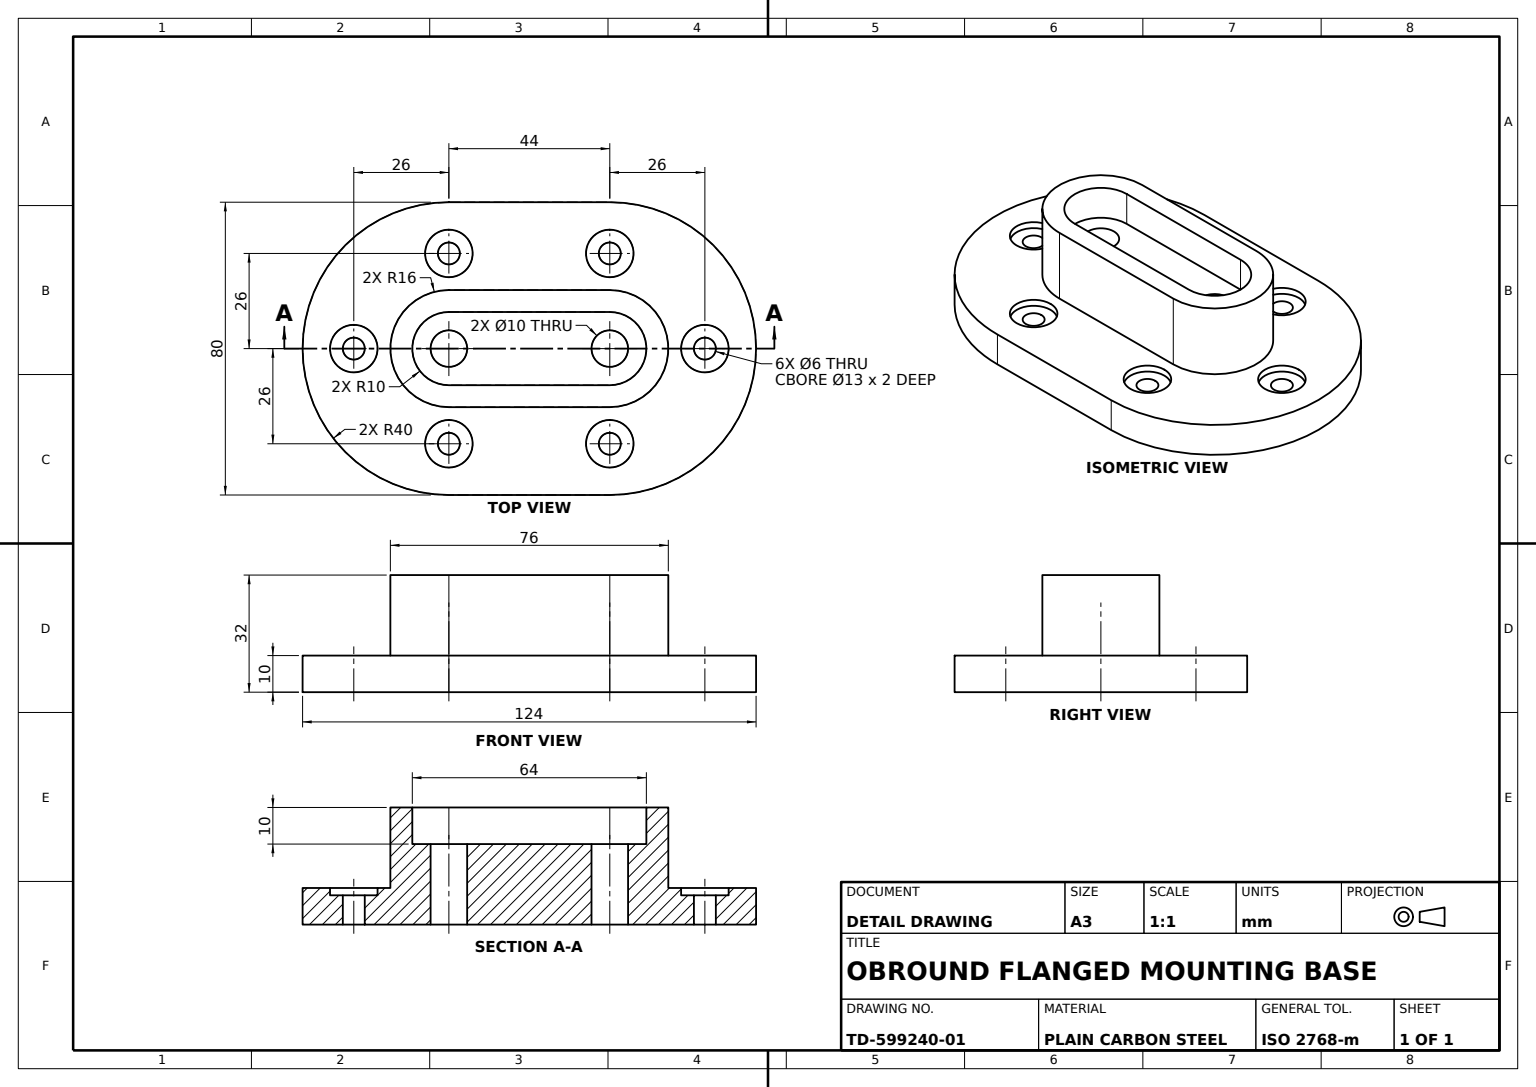
from build123d import *

# Parameters (mm, degrees)
BASE_FLANGE_DEPTH             = 10
SLOT_BOSS_DEPTH               = 22
SLOT_POCKET_DEPTH             = 10
SLOT_THROUGH_CUT_SKETCH_R     = 5
SLOT_THROUGH_CUT_DEPTH        = 53
COUNTERBORES_SKETCH_R         = 6.5
COUNTERBORES_6X_DEPTH_2_DEPTH = 2
MOUNTING_HOLES_SKETCH_R       = 3
MOUNTING_HOLES_6X_DEPTH       = 40


with BuildPart() as part:
    # Base Flange Sketch → Base Flange (new body)
    with BuildSketch(Plane(origin=(0, 0, 0), x_dir=(1, 0, 0), z_dir=(0, 1, 0))):
        with BuildLine():
            Line((-22, -40), (22, -40))
            ThreePointArc((22, -40), (62, 0), (22, 40))
            Line((22, 40), (-22, 40))
            ThreePointArc((-22, 40), (-62, 0), (-22, -40))
        make_face()
    extrude(amount=BASE_FLANGE_DEPTH)

    # Slot Boss Sketch → Slot Boss (add)
    with BuildSketch(Plane(origin=(0, 10, 0), x_dir=(1, 0, 0), z_dir=(0, 1, 0))):
        with BuildLine():
            Line((-22, 16), (22, 16))
            ThreePointArc((22, 16), (38, 0), (22, -16))
            Line((22, -16), (-22, -16))
            ThreePointArc((-22, -16), (-38, 0), (-22, 16))
        make_face()
    extrude(amount=SLOT_BOSS_DEPTH)

    # Slot Pocket Sketch → Slot Pocket (cut)
    with BuildSketch(Plane(origin=(0, 32, 0), x_dir=(1, 0, 0), z_dir=(0, 1, 0))):
        with BuildLine():
            Line((-22, 10), (22, 10))
            ThreePointArc((22, 10), (32, 0), (22, -10))
            Line((22, -10), (-22, -10))
            ThreePointArc((-22, -10), (-32, 0), (-22, 10))
        make_face()
    extrude(amount=-SLOT_POCKET_DEPTH, mode=Mode.SUBTRACT)

    # Slot Through Cut Sketch → Slot Through Cut (cut)
    with BuildSketch(Plane(origin=(0, 22, 0), x_dir=(1, 0, 0), z_dir=(0, 1, 0))):
        with Locations(Location((22, 0, 0), (0, 0, 270))):
            Circle(SLOT_THROUGH_CUT_SKETCH_R)
        with Locations(Location((-22, 0, 0), (0, 0, 270))):
            Circle(SLOT_THROUGH_CUT_SKETCH_R)
    extrude(amount=-SLOT_THROUGH_CUT_DEPTH, mode=Mode.SUBTRACT)

    # Counterbores Sketch → Counterbores 6x Depth 2 (cut)
    with BuildSketch(Plane(origin=(0, 10, 0), x_dir=(1, 0, 0), z_dir=(0, 1, 0))):
        with Locations(Location((48, 0, 0), (0, 0, 270))):
            Circle(COUNTERBORES_SKETCH_R)
        with Locations(Location((22, 26, 0), (0, 0, 270))):
            Circle(COUNTERBORES_SKETCH_R)
        with Locations(Location((-22, 26, 0), (0, 0, 270))):
            Circle(COUNTERBORES_SKETCH_R)
        with Locations(Location((-48, 0, 0), (0, 0, 270))):
            Circle(COUNTERBORES_SKETCH_R)
        with Locations(Location((-22, -26, 0), (0, 0, 270))):
            Circle(COUNTERBORES_SKETCH_R)
        with Locations(Location((22, -26, 0), (0, 0, 270))):
            Circle(COUNTERBORES_SKETCH_R)
    extrude(amount=-COUNTERBORES_6X_DEPTH_2_DEPTH, mode=Mode.SUBTRACT)

    # Mounting Holes Sketch → Mounting Holes 6x (cut)
    with BuildSketch(Plane(origin=(0, 8, 0), x_dir=(1, 0, 0), z_dir=(0, 1, 0))):
        with Locations(Location((48, 0, 0), (0, 0, 270))):
            Circle(MOUNTING_HOLES_SKETCH_R)
        with Locations(Location((22, -26, 0), (0, 0, 270))):
            Circle(MOUNTING_HOLES_SKETCH_R)
        with Locations(Location((-22, -26, 0), (0, 0, 270))):
            Circle(MOUNTING_HOLES_SKETCH_R)
        with Locations(Location((-48, 0, 0), (0, 0, 270))):
            Circle(MOUNTING_HOLES_SKETCH_R)
        with Locations(Location((-22, 26, 0), (0, 0, 270))):
            Circle(MOUNTING_HOLES_SKETCH_R)
        with Locations(Location((22, 26, 0), (0, 0, 270))):
            Circle(MOUNTING_HOLES_SKETCH_R)
    extrude(amount=-MOUNTING_HOLES_6X_DEPTH, mode=Mode.SUBTRACT)


solid = part.part
